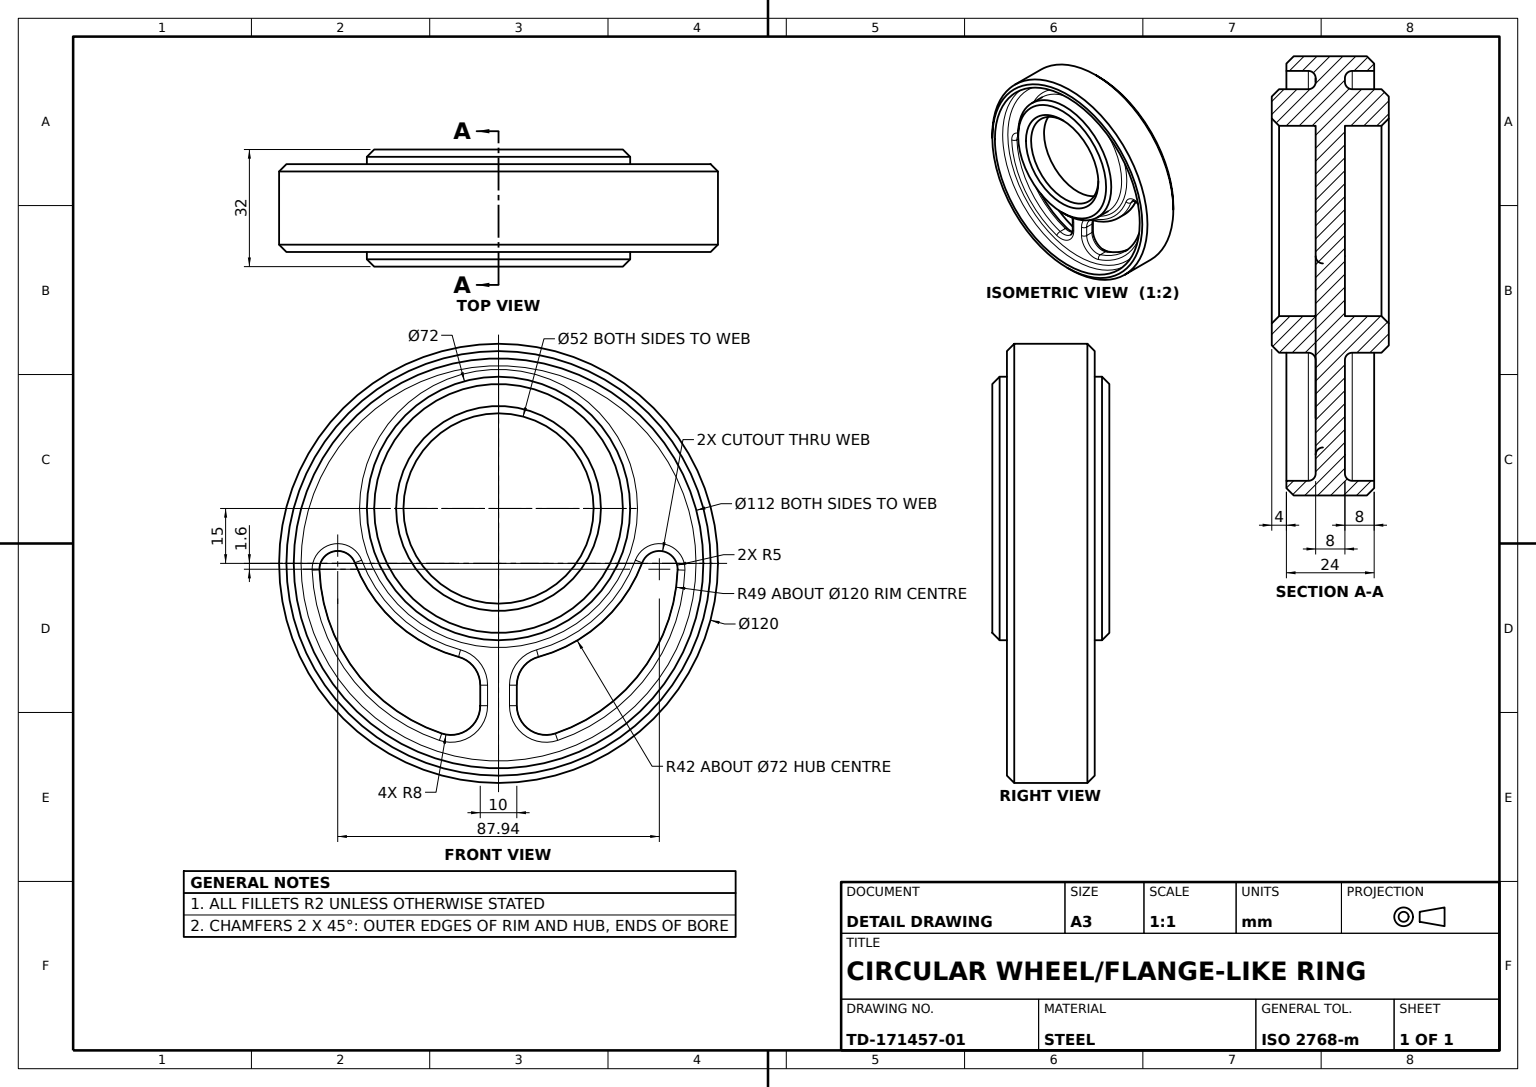
from build123d import *

# Parameters (mm, degrees)
DISC_RING_PROFILES_SKETCH_R   = 56
DISC_RING_PROFILES_SKETCH_R_2 = 36
DISC_RING_PROFILES_SKETCH_R_3 = 26
BASE_WEB_8MM_DEPTH            = 4
SKETCH3_3_R                   = 60
SKETCH3_3_R_2                 = 56
HUB_RING_24MM_DEPTH           = 12
SKETCH3_4_R                   = 36
SKETCH3_4_R_2                 = 26
OUTER_RIM_32MM_DEPTH          = 16
WEB_CUTOUTS_DEPTH             = 17
WEB_EDGE_FILLET_R2_R          = 2
RING_EDGE_CHAMFERS_2X45_SIZE  = 2


with BuildPart() as part:
    # Disc Ring Profiles Sketch → Base Web 8mm (new, symmetric)
    # profile 1 of 3: a face of its own
    with BuildSketch(Plane.XY):
        Circle(DISC_RING_PROFILES_SKETCH_R)
        with Locations((0, -15)):
            Circle(DISC_RING_PROFILES_SKETCH_R_2, mode=Mode.SUBTRACT)
    # profile 2 of 3: a face of its own
    with BuildSketch(Plane.XY):
        with Locations((0, -15)):
            Circle(DISC_RING_PROFILES_SKETCH_R_2)
        with Locations((0, -15)):
            Circle(DISC_RING_PROFILES_SKETCH_R_3, mode=Mode.SUBTRACT)
    # profile 3 of 3: a face of its own
    with BuildSketch(Plane.XY):
        with Locations((0, -15)):
            Circle(DISC_RING_PROFILES_SKETCH_R_3)
    extrude(amount=BASE_WEB_8MM_DEPTH, both=True)

    # Sketch3_3 → Hub Ring 24mm (add, symmetric)
    with BuildSketch(Plane.XY):
        Circle(SKETCH3_3_R)
        Circle(SKETCH3_3_R_2, mode=Mode.SUBTRACT)
    extrude(amount=HUB_RING_24MM_DEPTH, both=True)

    # Sketch3_4 → Outer Rim 32mm (add, symmetric)
    with BuildSketch(Plane.XY):
        with Locations((0, -15)):
            Circle(SKETCH3_4_R)
        with Locations((0, -15)):
            Circle(SKETCH3_4_R_2, mode=Mode.SUBTRACT)
    extrude(amount=OUTER_RIM_32MM_DEPTH, both=True)

    # Web Cutouts Sketch → Web Cutouts (cut, symmetric)
    with BuildSketch(Plane.XY):
        with BuildLine():
            Line((-5, 33.280430818), (-5, 38.88444419))
            ThreePointArc((-5, 38.88444419), (-8.325210322, 45.37646556), (-15.536585366, 46.471652813))
            ThreePointArc((-15.536585366, 46.471652813), (-39.236367993, 29.351446757), (-48.967592589, 1.781818182))
            ThreePointArc((-48.967592589, 1.781818182), (-44.957757013, -3.301643825), (-39.293144205, -0.165957447))
            ThreePointArc((-39.293144205, -0.165957447), (-28.208847937, 16.11689088), (-10.92, 25.555561887))
            ThreePointArc((-10.92, 25.555561887), (-6.650196853, 28.414220794), (-5, 33.280430818))
        make_face()
        with BuildLine():
            ThreePointArc((15.536585366, 46.471652813), (39.236367993, 29.351446757), (48.967592589, 1.781818182))
            ThreePointArc((48.967592589, 1.781818182), (44.957757013, -3.301643825), (39.293144205, -0.165957447))
            ThreePointArc((39.293144205, -0.165957447), (28.208847937, 16.11689088), (10.92, 25.555561887))
            ThreePointArc((10.92, 25.555561887), (6.650196853, 28.414220794), (5, 33.280430818))
            Line((5, 33.280430818), (5, 38.88444419))
            ThreePointArc((5, 38.88444419), (8.325210322, 45.37646556), (15.536585366, 46.471652813))
        make_face()
    extrude(amount=WEB_CUTOUTS_DEPTH, both=True, mode=Mode.SUBTRACT)

    # Web Edge Fillet R2
    web_edge_fillet_r2_edges = [part.edges().sort_by_distance(p)[0] for p in [
        (-36, -15, -4),
        (-36, -15, 4),
        (-56, 0, -4),
        (8.325210322, 45.37646556, -4),
        (5, 36.082437504, -4),
        (6.650196853, 28.414220794, -4),
        (28.208847937, 16.11689088, -4),
        (44.957757013, -3.301643825, -4),
        (39.236367993, 29.351446757, -4),
        (-8.325210322, 45.37646556, -4),
        (-39.236367993, 29.351446757, -4),
        (-44.957757013, -3.301643825, -4),
        (-28.208847937, 16.11689088, -4),
        (-6.650196853, 28.414220794, -4),
        (-5, 36.082437504, -4),
        (-5, 36.082437504, 4),
        (-6.650196853, 28.414220794, 4),
        (-28.208847937, 16.11689088, 4),
        (-44.957757013, -3.301643825, 4),
        (-39.236367993, 29.351446757, 4),
        (-8.325210322, 45.37646556, 4),
        (39.236367993, 29.351446757, 4),
        (44.957757013, -3.301643825, 4),
        (28.208847937, 16.11689088, 4),
        (6.650196853, 28.414220794, 4),
        (5, 36.082437504, 4),
        (8.325210322, 45.37646556, 4),
        (-56, 0, 4),
    ]]
    fillet(web_edge_fillet_r2_edges, radius=WEB_EDGE_FILLET_R2_R)

    # Ring Edge Chamfers 2x45
    ring_edge_chamfers_2x45_edges = [part.edges().sort_by_distance(p)[0] for p in [
        (-36, -15, -16),
        (-26, -15, 16),
        (-36, -15, 16),
        (-26, -15, -16),
        (-60, 0, -12),
        (-60, 0, 12),
    ]]
    chamfer(ring_edge_chamfers_2x45_edges, length=RING_EDGE_CHAMFERS_2X45_SIZE)


solid = part.part
